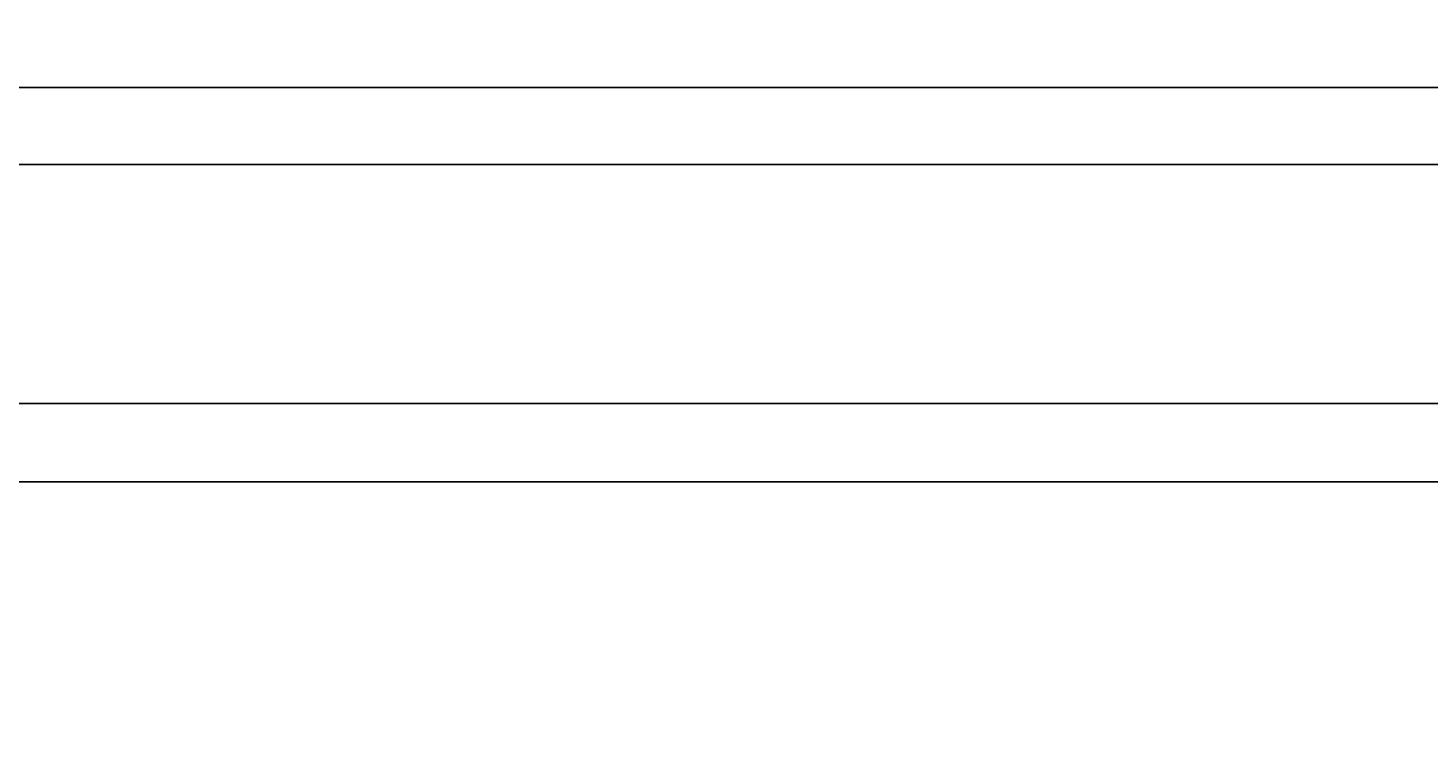
# Model space of a CAD drawing. Units: inches. Extents: x 35362 to 73946, y 43607 to 67532.
# Tile 9 of 134: x 42029 to 43509, y 46919 to 47688. Entities that reach past the tile are written whole.
import ezdxf

# ---------------------------------------------------------------- set-up
doc = ezdxf.new("R2010")
doc.units = ezdxf.units.IN
doc.header["$MEASUREMENT"] = 0
doc.layers.add('A-ANNO-DIMS', color=2, linetype='Continuous', lineweight=18)
doc.styles.get("Standard").update_dxf_attribs({"font": 'arial.ttf'})
doc.dimstyles.get("Standard").update_dxf_attribs({"dimtxt": 0.18, "dimasz": 0.18, "dimexe": 0.18, "dimexo": 0.0625, "dimgap": 0.09, "dimtad": 0, "dimtih": 1, "dimtoh": 1, "dimdec": 4, "dimzin": 0, "dimdsep": 46, "dimtxsty": 'Standard', "dimcen": 0.09, "dimadec": 0, "dimazin": 0, "dimtfac": 1, "dimtdec": 4, "dimtofl": 0, "dimtmove": 0, "dimatfit": 3, "dimfxl": 1, "dimtolj": 1, "dimtzin": 0, "dimarcsym": 0})

# ---------------------------------------------------------------- blocks, each defined once
blk = doc.blocks.new('*D43')
at = {"layer": 'A-ANNO-DIMS', "color": 0, "lineweight": -2, "transparency": 16777216}
for p, q in [((62004.7, 47625.2), (35361.8, 47625.2)), ((35361.9, 47625), (35361.9, 47416.9)), ((35361.9, 47208.4), (35361.9, 47416.5)), ((62004.7, 47208.2), (35361.8, 47208.2))]:
    blk.add_line(p, q, dxfattribs=at)
at = {"layer": 'A-ANNO-DIMS', "color": 0, "transparency": 16777216}
for points in [[(35361.9, 47625), (35362, 47625), (35361.9, 47625.2)], [(35361.9, 47208.4), (35362, 47208.4), (35361.9, 47208.2)]]:
    blk.add_solid(points, dxfattribs=at)
at = {"layer": 'Defpoints', "color": 0, "transparency": 16777216}
for p in [(62004.7, 47625.2), (35361.9, 47208.2), (62004.7, 47208.2)]:
    blk.add_point(p, dxfattribs=at)
at = {"layer": 'A-ANNO-DIMS', "color": 0, "transparency": 16777216, "insert": (35361.9, 47416.7), "char_height": 0.18, "attachment_point": 5}
blk.add_mtext('\\A1;416.9', dxfattribs=at)
blk = doc.blocks.new('*D67')
at = {"layer": 'A-ANNO-DIMS', "color": 0, "lineweight": -2, "transparency": 16777216}
for p, q in [((56873.5, 53351.5), (35361.8, 53351.5)), ((35361.9, 53351.3), (35361.9, 49400.9)), ((35361.9, 45450.1), (35361.9, 49400.5)), ((53793.6, 45449.9), (35361.8, 45449.9))]:
    blk.add_line(p, q, dxfattribs=at)
at = {"layer": 'A-ANNO-DIMS', "color": 0, "transparency": 16777216}
for points in [[(35361.9, 53351.3), (35362, 53351.3), (35361.9, 53351.5)], [(35361.9, 45450.1), (35362, 45450.1), (35361.9, 45449.9)]]:
    blk.add_solid(points, dxfattribs=at)
at = {"layer": 'Defpoints', "color": 0, "transparency": 16777216}
for p in [(35361.9, 53351.5), (56873.6, 53351.5), (53793.6, 45449.9)]:
    blk.add_point(p, dxfattribs=at)
at = {"layer": 'A-ANNO-DIMS', "color": 0, "transparency": 16777216, "insert": (35361.9, 49400.7), "char_height": 0.18, "attachment_point": 5}
blk.add_mtext('\\A1;7901.6', dxfattribs=at)
blk = doc.blocks.new('*D87')
at = {"layer": 'A-ANNO-DIMS', "color": 0, "lineweight": -2, "transparency": 16777216}
for p, q in [((52362.5, 48318.3), (35361.8, 48318.3)), ((35361.9, 48318.1), (35361.9, 47931.4)), ((35361.9, 47544.3), (35361.9, 47931)), ((52362.5, 47544.1), (35361.8, 47544.1))]:
    blk.add_line(p, q, dxfattribs=at)
at = {"layer": 'A-ANNO-DIMS', "color": 0, "transparency": 16777216}
for points in [[(35361.9, 48318.1), (35362, 48318.1), (35361.9, 48318.3)], [(35361.9, 47544.3), (35362, 47544.3), (35361.9, 47544.1)]]:
    blk.add_solid(points, dxfattribs=at)
at = {"layer": 'Defpoints', "color": 0, "transparency": 16777216}
for p in [(35361.9, 48318.3), (52362.6, 48318.3), (52362.6, 47544.1)]:
    blk.add_point(p, dxfattribs=at)
at = {"layer": 'A-ANNO-DIMS', "color": 0, "transparency": 16777216, "insert": (35361.9, 47931.2), "char_height": 0.18, "attachment_point": 5}
blk.add_mtext('\\A1;774.1', dxfattribs=at)
blk = doc.blocks.new('*D90')
at = {"layer": 'A-ANNO-DIMS', "color": 0, "lineweight": -2, "transparency": 16777216}
for p, q in [((53707.7, 47291.3), (35361.8, 47291.3)), ((35361.9, 47291.1), (35361.9, 46710.3)), ((35361.9, 46129.1), (35361.9, 46709.9)), ((53793.6, 46128.9), (35361.8, 46128.9))]:
    blk.add_line(p, q, dxfattribs=at)
at = {"layer": 'A-ANNO-DIMS', "color": 0, "transparency": 16777216}
for points in [[(35361.9, 47291.1), (35362, 47291.1), (35361.9, 47291.3)], [(35361.9, 46129.1), (35362, 46129.1), (35361.9, 46128.9)]]:
    blk.add_solid(points, dxfattribs=at)
at = {"layer": 'Defpoints', "color": 0, "transparency": 16777216}
for p in [(53707.8, 47291.3), (35361.9, 46128.9), (53793.6, 46128.9)]:
    blk.add_point(p, dxfattribs=at)
at = {"layer": 'A-ANNO-DIMS', "color": 0, "transparency": 16777216, "insert": (35361.9, 46710.1), "char_height": 0.18, "attachment_point": 5}
blk.add_mtext('\\A1;1162.4', dxfattribs=at)

msp = doc.modelspace()

# ---------------------------------------------------------------- dimensions: what is measured, and where the dimension line sits
at = {"layer": 'A-ANNO-DIMS'}
for base, p1, p2, picture, middle in [((35361.949, 53351.529), (53793.638, 45449.894), (56873.602, 53351.529), '*D67', (35361.949, 49400.712)), ((35361.949, 48318.269), (52362.557, 47544.134), (52362.557, 48318.269), '*D87', (35361.949, 47931.201)), ((35361.949, 47208.25), (62004.728, 47625.181), (62004.728, 47208.25), '*D43', (35361.949, 47416.715)), ((35361.949, 46128.878), (53707.781, 47291.285), (53793.638, 46128.878), '*D90', (35361.949, 46710.081))]:
    dim = msp.add_linear_dim(base=base, p1=p1, p2=p2, angle=90, dimstyle='Standard', override={"dimdec": 1, "dimlfac": 1, "dimrnd": 0, "dimzin": 0, "dimdsep": 46, "dimlunit": 2}, dxfattribs=at)
    dim.commit()
    dim.dimension.update_dxf_attribs({"geometry": picture, "text_midpoint": middle})

doc.saveas('drawing.dxf')
